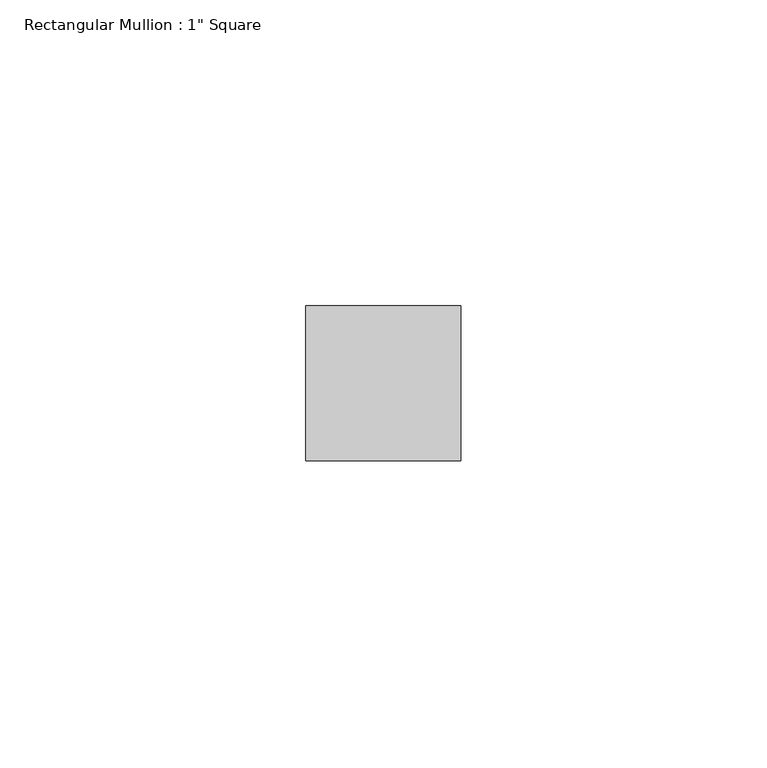
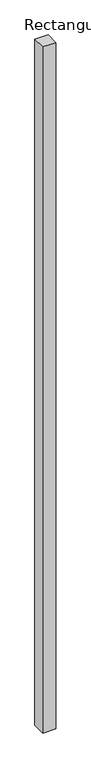
"""IFC4 building model written with IfcOpenShell, lengths in millimetres: member geometry."""

from ifc_helpers import new_model, si_unit, frame, origin, place, context, project, spatial, polyline, outline, extrude, source, transform, mapped, element, save


def member_84ecdb2b(model_context):
    return source(origin(), model_context, "Body", "SweptSolid", [
        extrude(outline(polyline([(12.7, 12.7), (12.7, -12.7), (-12.7, -12.7), (-12.7, 12.7), (12.7, 12.7)])), frame((0.0, 0.0, -1384.3), z_axis=(0.0, 0.0, 1.0), x_axis=(1.0, 0.0, 0.0)), (0.0, 0.0, 1.0), 1384.3),
    ])


if __name__ == "__main__":
    model = new_model("IFC4")
    model_context = context("Model", 3, world=origin())
    ifc_project = project(units=[si_unit("LENGTHUNIT", "METRE", prefix="MILLI")], contexts=[model_context])
    site = spatial("IfcSite", under=ifc_project)
    building = spatial("IfcBuilding", under=site)
    placement = place(None, origin())
    member_shape = member_84ecdb2b(model_context)
    element("IfcMember", 1, ObjectType="Rectangular Mullion : 1\" Square", at=placement, inside=building, context=model_context, shape_type="MappedRepresentation", body=[
        mapped(member_shape, transform((0.0, 0.0, 0.0), x_axis=(1.0, 0.0, 0.0), y_axis=(0.0, 1.0, 0.0), z_axis=(0.0, 0.0, 1.0))),
    ])
    save(model, "model.ifc")

# Revit data of these elements
# Type "Rectangular Mullion : 1\" Square"
#   built-in parameter 1007304 = 0.0833333 (stored number, unit not read)
#   built-in parameter 1007301 = 0.0416667 (stored number, unit not read)
#   built-in parameter 1007300 = 0.0416667 (stored number, unit not read)
